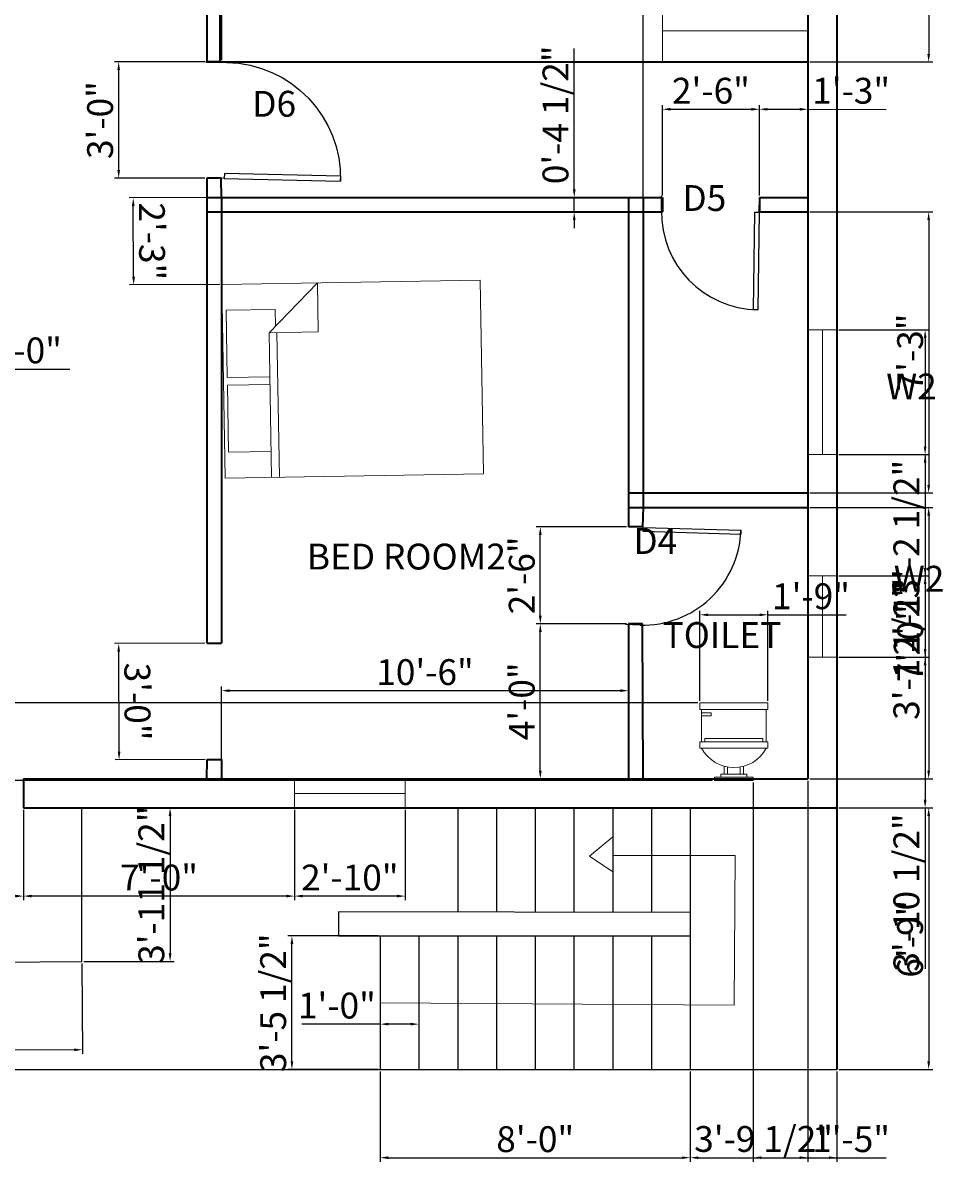
# Model space of a CAD drawing. Units: inches. Extents: x 56 to 631, y 587 to 1198.
# Tile 2 of 3: x 344 to 631, y 587 to 946. Entities that reach past the tile are written whole.
import ezdxf

# ---------------------------------------------------------------- set-up
doc = ezdxf.new("R2010")
doc.units = ezdxf.units.IN
for name, color, linetype, lineweight in [('A-ANNO-DIMS', 2, 'Continuous', 18), ('A-ANNO-SYMB', 2, 'Continuous', 13), ('A-ANNO-TEXT', 7, 'Continuous', 18), ('A-AREA-IDEN', 7, 'Continuous', 25), ('A-DOOR', 3, 'Continuous', 25), ('A-FLOR-CASE', 9, 'Continuous', 18), ('A-FLOR-FIXT', 9, 'Continuous', 18), ('A-FLOR-OTLN', 7, 'Continuous', 25), ('A-FLOR-STRS', 7, 'Continuous', 25), ('A-FURN', 8, 'Continuous', 18), ('A-GLAZ', 4, 'Continuous', 18), ('WALL', 7, 'Continuous', 35)]:
    doc.layers.add(name, color=color, linetype=linetype, lineweight=lineweight)
doc.styles.get("Standard").update_dxf_attribs({"font": 'arial.ttf', "height": 8})
doc.dimstyles.new('ISO-25', dxfattribs={"dimtxt": 2.5, "dimasz": 2.5, "dimexe": 1.25, "dimexo": 0.625, "dimtad": 1, "dimdec": 1, "dimlunit": 3, "dimtxsty": 'Standard', "dimcen": 2.5, "dimadec": 0, "dimazin": 0, "dimtfac": 1, "dimtdec": 1, "dimtmove": 0, "dimatfit": 3, "dimfxl": 1, "dimarcsym": 0})

# ---------------------------------------------------------------- blocks, each defined once
blk = doc.blocks.new('*U2')
for p, q in [((-40, 0), (-40, 6)), ((0, 0), (0, 6))]:
    blk.add_line(p, q)
blk.add_lwpolyline([(0, 0), (0, -40), (-1.75, -40), (-1.75, 0)], close=True)
blk.add_arc((0, 0), 40, 180, 270)
blk = doc.blocks.new('*U3')
for p, q in [((0, 0), (0, -6)), ((40, 0), (40, -6))]:
    blk.add_line(p, q)
blk.add_lwpolyline([(0, 0), (0, 40), (1.75, 40), (1.75, 0)], close=True)
blk.add_arc((0, 0), 40, 0, 90)
blk = doc.blocks.new('Bed - Queen')
for p, q in [((0, -80.00003), (0, 0)), ((0, 0), (59.99999, 0)), ((59.99999, 0), (59.99999, -80.00003)), ((7.99999, -1.2), (28.79998, -1.2)), ((7.99999, -14.4), (7.99999, -1.2)), ((28.79998, -1.2), (28.79998, -14.4)), ((31.19999, -1.2), (51.99999, -1.2)), ((31.19999, -14.4), (31.19999, -1.2)), ((51.99999, -1.2), (51.99999, -16.4)), ((0, -14.4), (44.8, -14.4)), ((44.8, -16.8), (0, -16.8)), ((59.99999, -29.6), (44.8, -14.4)), ((44.8, -14.4), (44.8, -29.6)), ((51.99999, -16.4), (46.79936, -16.4)), ((44.8, -29.6), (59.99999, -29.6)), ((59.99999, -80.00003), (0, -80.00003))]:
    blk.add_line(p, q)
blk = doc.blocks.new('*U10')
for p, q in [((-10, 22), (-10, 12)), ((10, 12), (10, 22)), ((-10, 21), (-7, 21)), ((-7, 20), (-10, 20)), ((-7, 21), (-7, 20)), ((10.5, 12), (-10.5, 12)), ((-10.5, 10), (-10.5, 12)), ((9, 13), (-9, 13)), ((-9, 13), (-9, 12)), ((9, 12), (9, 13)), ((10.5, 12), (10.5, 10)), ((10.5, 10), (-10.5, 10)), ((-3, 4.4065), (-3, 2)), ((-2, 2), (-2, 4.1658)), ((2, 4.1658), (2, 2)), ((3, 2), (3, 4.4065)), ((4, 2), (-4, 2)), ((-4, 2), (-4, 1)), ((4, 1), (4, 2))]:
    blk.add_line(p, q)
for points in [[(10.5, 22), (10.5, 24), (-10.5, 24), (-10.5, 22)], [(6, 0), (6, 1), (-6, 1), (-6, 0)]]:
    blk.add_lwpolyline(points, close=True)
blk.add_arc((0, 15.3333), 11.3333, 208.0725, 331.9275)
blk = doc.blocks.new('*D17')
at = {"layer": 'A-ANNO-DIMS', "color": 0, "lineweight": -2, "transparency": 16777216}
for p, q in [((211.72, 847), (211.72, 837.38)), ((271.72, 847), (271.72, 837.38)), ((214.22, 838.63), (269.22, 838.63)), ((271.72, 838.63), (358.5, 838.63))]:
    blk.add_line(p, q, dxfattribs=at)
at = {"layer": 'A-ANNO-DIMS', "color": 0, "transparency": 16777216}
for points in [[(214.22, 839.05), (214.22, 838.21), (211.72, 838.63)], [(269.22, 839.05), (269.22, 838.21), (271.72, 838.63)]]:
    blk.add_solid(points, dxfattribs=at)
at = {"layer": 'Defpoints', "color": 0, "transparency": 16777216}
for p in [(211.72, 847.63), (271.72, 847.63), (271.72, 838.63)]:
    blk.add_point(p, dxfattribs=at)
at = {"layer": 'A-ANNO-DIMS', "color": 0, "transparency": 16777216, "insert": (316.36, 843.39), "char_height": 8, "attachment_point": 5}
blk.add_mtext('LOVESEAT 5\'-0"', dxfattribs=at)
blk = doc.blocks.new('*D24')
at = {"layer": 'A-ANNO-DIMS', "color": 0, "lineweight": -2, "transparency": 16777216}
for p, q in [((405.55, 934.28), (405.54, 962.2)), ((408.04, 960.95), (584.4, 961.04)), ((586.91, 934.37), (586.9, 962.3))]:
    blk.add_line(p, q, dxfattribs=at)
at = {"layer": 'A-ANNO-DIMS', "color": 0, "transparency": 16777216}
for points in [[(408.04, 961.37), (408.04, 960.54), (405.54, 960.95)], [(584.4, 961.46), (584.4, 960.63), (586.9, 961.05)]]:
    blk.add_solid(points, dxfattribs=at)
at = {"layer": 'Defpoints', "color": 0, "transparency": 16777216}
for p in [(586.9, 961.05), (405.55, 933.65), (586.92, 933.75)]:
    blk.add_point(p, dxfattribs=at)
at = {"layer": 'A-ANNO-DIMS', "color": 0, "transparency": 16777216, "insert": (496.22, 965.76), "char_height": 8, "attachment_point": 5, "rotation": 0.0297}
blk.add_mtext('15\'-1 1/2"', dxfattribs=at)
blk = doc.blocks.new('*D25')
at = {"layer": 'A-ANNO-DIMS', "color": 0, "lineweight": -2, "transparency": 16777216}
for p, q in [((405.42, 712.41), (405.42, 740.34)), ((407.92, 739.09), (528.92, 739.09)), ((531.42, 712.41), (531.42, 740.34))]:
    blk.add_line(p, q, dxfattribs=at)
at = {"layer": 'A-ANNO-DIMS', "color": 0, "transparency": 16777216}
for points in [[(407.92, 739.5), (407.92, 738.67), (405.42, 739.09)], [(528.92, 739.5), (528.92, 738.67), (531.42, 739.09)]]:
    blk.add_solid(points, dxfattribs=at)
at = {"layer": 'Defpoints', "color": 0, "transparency": 16777216}
for p in [(531.42, 739.09), (405.42, 711.79), (531.42, 711.79)]:
    blk.add_point(p, dxfattribs=at)
at = {"layer": 'A-ANNO-DIMS', "color": 0, "transparency": 16777216, "insert": (468.42, 743.79), "char_height": 8, "attachment_point": 5}
blk.add_mtext('10\'-6"', dxfattribs=at)
blk = doc.blocks.new('*D26')
at = {"layer": 'A-ANNO-DIMS', "color": 0, "lineweight": -2, "transparency": 16777216}
for p, q in [((535.92, 796.41), (535.92, 1113.84)), ((538.42, 1112.59), (584.42, 1112.59)), ((586.92, 796.41), (586.92, 1113.84))]:
    blk.add_line(p, q, dxfattribs=at)
at = {"layer": 'A-ANNO-DIMS', "color": 0, "transparency": 16777216}
for points in [[(538.42, 1113), (538.42, 1112.17), (535.92, 1112.59)], [(584.42, 1113), (584.42, 1112.17), (586.92, 1112.59)]]:
    blk.add_solid(points, dxfattribs=at)
at = {"layer": 'Defpoints', "color": 0, "transparency": 16777216}
for p in [(586.92, 1112.59), (535.92, 795.79), (586.92, 795.79)]:
    blk.add_point(p, dxfattribs=at)
at = {"layer": 'A-ANNO-DIMS', "color": 0, "transparency": 16777216, "insert": (561.42, 1117.3), "char_height": 8, "attachment_point": 5}
blk.add_mtext('4\'-3"', dxfattribs=at)
blk = doc.blocks.new('*D29')
at = {"layer": 'A-ANNO-DIMS', "color": 0, "lineweight": -2, "transparency": 16777216}
for p, q in [((596.54, 702.79), (625.57, 702.79)), ((624.32, 700.29), (624.32, 624.29)), ((596.54, 621.79), (625.57, 621.79))]:
    blk.add_line(p, q, dxfattribs=at)
at = {"layer": 'A-ANNO-DIMS', "color": 0, "transparency": 16777216}
for points in [[(623.9, 700.29), (624.74, 700.29), (624.32, 702.79)], [(623.9, 624.29), (624.74, 624.29), (624.32, 621.79)]]:
    blk.add_solid(points, dxfattribs=at)
at = {"layer": 'Defpoints', "color": 0, "transparency": 16777216}
for p in [(595.92, 702.79), (595.92, 621.79), (624.32, 621.79)]:
    blk.add_point(p, dxfattribs=at)
at = {"layer": 'A-ANNO-DIMS', "color": 0, "transparency": 16777216, "insert": (619.61, 662.29), "char_height": 8, "attachment_point": 5, "rotation": 90}
blk.add_mtext('6\'-9"', dxfattribs=at)
blk = doc.blocks.new('*D30')
at = {"layer": 'A-ANNO-DIMS', "color": 0, "lineweight": -2, "transparency": 16777216}
for p, q in [((587.54, 1076.29), (625.57, 1076.29)), ((624.32, 1073.79), (624.32, 936.25)), ((587.54, 933.75), (625.57, 933.75))]:
    blk.add_line(p, q, dxfattribs=at)
at = {"layer": 'A-ANNO-DIMS', "color": 0, "transparency": 16777216}
for points in [[(623.9, 1073.79), (624.74, 1073.79), (624.32, 1076.29)], [(623.9, 936.25), (624.74, 936.25), (624.32, 933.75)]]:
    blk.add_solid(points, dxfattribs=at)
at = {"layer": 'Defpoints', "color": 0, "transparency": 16777216}
for p in [(586.92, 1076.29), (586.92, 933.75), (624.32, 933.75)]:
    blk.add_point(p, dxfattribs=at)
at = {"layer": 'A-ANNO-DIMS', "color": 0, "transparency": 16777216, "insert": (619.56, 1005.02), "char_height": 8, "attachment_point": 5, "rotation": 90}
blk.add_mtext('11\'-10 1/2"', dxfattribs=at)
blk = doc.blocks.new('*D31')
at = {"layer": 'A-ANNO-DIMS', "color": 0, "lineweight": -2, "transparency": 16777216}
for p, q in [((587.54, 887.29), (625.57, 887.29)), ((624.32, 884.79), (624.32, 802.79)), ((587.54, 800.29), (625.57, 800.29))]:
    blk.add_line(p, q, dxfattribs=at)
at = {"layer": 'A-ANNO-DIMS', "color": 0, "transparency": 16777216}
for points in [[(623.9, 884.79), (624.74, 884.79), (624.32, 887.29)], [(623.9, 802.79), (624.74, 802.79), (624.32, 800.29)]]:
    blk.add_solid(points, dxfattribs=at)
at = {"layer": 'Defpoints', "color": 0, "transparency": 16777216}
for p in [(586.92, 887.29), (586.92, 800.29), (624.32, 800.29)]:
    blk.add_point(p, dxfattribs=at)
at = {"layer": 'A-ANNO-DIMS', "color": 0, "transparency": 16777216, "insert": (619.61, 843.79), "char_height": 8, "attachment_point": 5, "rotation": 90}
blk.add_mtext('7\'-3"', dxfattribs=at)
blk = doc.blocks.new('*D32')
at = {"layer": 'A-ANNO-DIMS', "color": 0, "lineweight": -2, "transparency": 16777216}
for p, q in [((587.54, 795.79), (625.57, 795.79)), ((624.32, 793.29), (624.32, 714.29)), ((587.54, 711.79), (625.57, 711.79))]:
    blk.add_line(p, q, dxfattribs=at)
at = {"layer": 'A-ANNO-DIMS', "color": 0, "transparency": 16777216}
for points in [[(623.9, 793.29), (624.74, 793.29), (624.32, 795.79)], [(623.9, 714.29), (624.74, 714.29), (624.32, 711.79)]]:
    blk.add_solid(points, dxfattribs=at)
at = {"layer": 'Defpoints', "color": 0, "transparency": 16777216}
for p in [(586.92, 795.79), (586.92, 711.79), (624.32, 711.79)]:
    blk.add_point(p, dxfattribs=at)
at = {"layer": 'A-ANNO-DIMS', "color": 0, "transparency": 16777216, "insert": (619.61, 753.79), "char_height": 8, "attachment_point": 5, "rotation": 90}
blk.add_mtext('7\'-0"', dxfattribs=at)
blk = doc.blocks.new('*D40')
at = {"layer": 'A-ANNO-DIMS', "color": 0, "lineweight": -2, "transparency": 16777216}
for p, q in [((296.18, 702.16), (296.18, 674.24)), ((344.18, 702.16), (344.18, 674.24)), ((341.68, 675.49), (298.68, 675.49))]:
    blk.add_line(p, q, dxfattribs=at)
at = {"layer": 'A-ANNO-DIMS', "color": 0, "transparency": 16777216}
for points in [[(298.68, 675.9), (298.68, 675.07), (296.18, 675.49)], [(341.68, 675.9), (341.68, 675.07), (344.18, 675.49)]]:
    blk.add_solid(points, dxfattribs=at)
at = {"layer": 'Defpoints', "color": 0, "transparency": 16777216}
for p in [(296.18, 702.79), (344.18, 702.79), (296.18, 675.49)]:
    blk.add_point(p, dxfattribs=at)
at = {"layer": 'A-ANNO-DIMS', "color": 0, "transparency": 16777216, "insert": (320.18, 680.19), "char_height": 8, "attachment_point": 5}
blk.add_mtext('4\'-0"', dxfattribs=at)
blk = doc.blocks.new('*D41')
at = {"layer": 'A-ANNO-DIMS', "color": 0, "lineweight": -2, "transparency": 16777216}
for p, q in [((344.18, 702.16), (344.18, 674.24)), ((428.03, 702.16), (428.03, 674.24)), ((425.53, 675.49), (346.68, 675.49))]:
    blk.add_line(p, q, dxfattribs=at)
at = {"layer": 'A-ANNO-DIMS', "color": 0, "transparency": 16777216}
for points in [[(346.68, 675.9), (346.68, 675.07), (344.18, 675.49)], [(425.53, 675.9), (425.53, 675.07), (428.03, 675.49)]]:
    blk.add_solid(points, dxfattribs=at)
at = {"layer": 'Defpoints', "color": 0, "transparency": 16777216}
for p in [(344.18, 702.79), (428.03, 702.79), (344.18, 675.49)]:
    blk.add_point(p, dxfattribs=at)
at = {"layer": 'A-ANNO-DIMS', "color": 0, "transparency": 16777216, "insert": (386.11, 680.19), "char_height": 8, "attachment_point": 5}
blk.add_mtext('7\'-0"', dxfattribs=at)
blk = doc.blocks.new('*D42')
at = {"layer": 'A-ANNO-DIMS', "color": 0, "lineweight": -2, "transparency": 16777216}
for p, q in [((428.03, 702.16), (428.03, 674.24)), ((462.27, 702.16), (462.27, 674.24)), ((459.77, 675.49), (430.53, 675.49))]:
    blk.add_line(p, q, dxfattribs=at)
at = {"layer": 'A-ANNO-DIMS', "color": 0, "transparency": 16777216}
for points in [[(430.53, 675.9), (430.53, 675.07), (428.03, 675.49)], [(459.77, 675.9), (459.77, 675.07), (462.27, 675.49)]]:
    blk.add_solid(points, dxfattribs=at)
at = {"layer": 'Defpoints', "color": 0, "transparency": 16777216}
for p in [(428.03, 702.79), (462.27, 702.79), (428.03, 675.49)]:
    blk.add_point(p, dxfattribs=at)
at = {"layer": 'A-ANNO-DIMS', "color": 0, "transparency": 16777216, "insert": (445.15, 680.19), "char_height": 8, "attachment_point": 5}
blk.add_mtext('2\'-10"', dxfattribs=at)
blk = doc.blocks.new('*D51')
at = {"layer": 'A-ANNO-DIMS', "color": 0, "lineweight": -2, "transparency": 16777216}
for p, q in [((596.54, 774.6), (624.47, 774.6)), ((623.22, 772.1), (623.22, 751.96)), ((596.54, 749.46), (624.47, 749.46))]:
    blk.add_line(p, q, dxfattribs=at)
at = {"layer": 'A-ANNO-DIMS', "color": 0, "transparency": 16777216}
for points in [[(622.8, 772.1), (623.63, 772.1), (623.22, 774.6)], [(622.8, 751.96), (623.63, 751.96), (623.22, 749.46)]]:
    blk.add_solid(points, dxfattribs=at)
at = {"layer": 'Defpoints', "color": 0, "transparency": 16777216}
for p in [(595.92, 774.6), (595.92, 749.46), (623.22, 749.46)]:
    blk.add_point(p, dxfattribs=at)
at = {"layer": 'A-ANNO-DIMS', "color": 0, "transparency": 16777216, "insert": (618.57, 762.03), "char_height": 8, "attachment_point": 5, "rotation": 90}
blk.add_mtext('2\'-1"', dxfattribs=at)
blk = doc.blocks.new('*D52')
at = {"layer": 'A-ANNO-DIMS', "color": 0, "lineweight": -2, "transparency": 16777216}
for p, q in [((596.54, 749.46), (624.47, 749.46)), ((623.22, 746.96), (623.22, 705.29)), ((596.54, 702.79), (624.47, 702.79)), ((623.22, 702.79), (623.22, 652.92))]:
    blk.add_line(p, q, dxfattribs=at)
at = {"layer": 'A-ANNO-DIMS', "color": 0, "transparency": 16777216}
for points in [[(622.8, 746.96), (623.63, 746.96), (623.22, 749.46)], [(622.8, 705.29), (623.63, 705.29), (623.22, 702.79)]]:
    blk.add_solid(points, dxfattribs=at)
at = {"layer": 'Defpoints', "color": 0, "transparency": 16777216}
for p in [(595.92, 749.46), (595.92, 702.79), (623.22, 702.79)]:
    blk.add_point(p, dxfattribs=at)
at = {"layer": 'A-ANNO-DIMS', "color": 0, "transparency": 16777216, "insert": (618.45, 676.6), "char_height": 8, "attachment_point": 5, "rotation": 90}
blk.add_mtext('3\'-10 1/2"', dxfattribs=at)
blk = doc.blocks.new('*D53')
at = {"layer": 'A-ANNO-DIMS', "color": 0, "lineweight": -2, "transparency": 16777216}
for p, q in [((596.54, 812.18), (624.47, 812.18)), ((623.22, 809.68), (623.22, 777.1)), ((596.54, 774.6), (624.47, 774.6)), ((623.22, 774.6), (623.22, 730.95))]:
    blk.add_line(p, q, dxfattribs=at)
at = {"layer": 'A-ANNO-DIMS', "color": 0, "transparency": 16777216}
for points in [[(622.8, 809.68), (623.63, 809.68), (623.22, 812.18)], [(622.8, 777.1), (623.63, 777.1), (623.22, 774.6)]]:
    blk.add_solid(points, dxfattribs=at)
at = {"layer": 'Defpoints', "color": 0, "transparency": 16777216}
for p in [(595.92, 812.18), (595.92, 774.6), (623.22, 774.6)]:
    blk.add_point(p, dxfattribs=at)
at = {"layer": 'A-ANNO-DIMS', "color": 0, "transparency": 16777216, "insert": (618.45, 751.53), "char_height": 8, "attachment_point": 5, "rotation": 90}
blk.add_mtext('3\'-1 1/2"', dxfattribs=at)
blk = doc.blocks.new('*D54')
at = {"layer": 'A-ANNO-DIMS', "color": 0, "lineweight": -2, "transparency": 16777216}
for p, q in [((596.54, 850.81), (624.47, 850.81)), ((623.22, 848.31), (623.22, 814.68)), ((596.54, 812.18), (624.47, 812.18)), ((623.22, 812.18), (623.22, 768.52))]:
    blk.add_line(p, q, dxfattribs=at)
at = {"layer": 'A-ANNO-DIMS', "color": 0, "transparency": 16777216}
for points in [[(622.8, 848.31), (623.63, 848.31), (623.22, 850.81)], [(622.8, 814.68), (623.63, 814.68), (623.22, 812.18)]]:
    blk.add_solid(points, dxfattribs=at)
at = {"layer": 'Defpoints', "color": 0, "transparency": 16777216}
for p in [(595.92, 850.81), (595.92, 812.18), (623.22, 812.18)]:
    blk.add_point(p, dxfattribs=at)
at = {"layer": 'A-ANNO-DIMS', "color": 0, "transparency": 16777216, "insert": (618.45, 789.1), "char_height": 8, "attachment_point": 5, "rotation": 90}
blk.add_mtext('3\'-2 1/2"', dxfattribs=at)
blk = doc.blocks.new('*D55')
at = {"layer": 'A-ANNO-DIMS', "color": 0, "lineweight": -2, "transparency": 16777216}
for p, q in [((541.92, 892.42), (541.92, 920.34)), ((544.42, 919.09), (569.42, 919.09)), ((571.92, 892.42), (571.92, 920.34))]:
    blk.add_line(p, q, dxfattribs=at)
at = {"layer": 'A-ANNO-DIMS', "color": 0, "transparency": 16777216}
for points in [[(544.42, 919.51), (544.42, 918.68), (541.92, 919.09)], [(569.42, 919.51), (569.42, 918.68), (571.92, 919.09)]]:
    blk.add_solid(points, dxfattribs=at)
at = {"layer": 'Defpoints', "color": 0, "transparency": 16777216}
for p in [(571.92, 919.09), (541.92, 891.79), (571.92, 891.79)]:
    blk.add_point(p, dxfattribs=at)
at = {"layer": 'A-ANNO-DIMS', "color": 0, "transparency": 16777216, "insert": (556.92, 923.8), "char_height": 8, "attachment_point": 5}
blk.add_mtext('2\'-6"', dxfattribs=at)
blk = doc.blocks.new('*D56')
at = {"layer": 'A-ANNO-DIMS', "color": 0, "lineweight": -2, "transparency": 16777216}
for p, q in [((571.92, 892.42), (571.93, 920.34)), ((574.43, 919.09), (584.43, 919.09)), ((586.92, 892.41), (586.93, 920.34)), ((586.93, 919.09), (611.19, 919.07))]:
    blk.add_line(p, q, dxfattribs=at)
at = {"layer": 'A-ANNO-DIMS', "color": 0, "transparency": 16777216}
for points in [[(574.43, 919.51), (574.43, 918.68), (571.93, 919.09)], [(584.43, 919.5), (584.43, 918.67), (586.93, 919.09)]]:
    blk.add_solid(points, dxfattribs=at)
at = {"layer": 'Defpoints', "color": 0, "transparency": 16777216}
for p in [(586.93, 919.09), (571.92, 891.79), (586.92, 891.79)]:
    blk.add_point(p, dxfattribs=at)
at = {"layer": 'A-ANNO-DIMS', "color": 0, "transparency": 16777216, "insert": (600.32, 923.79), "char_height": 8, "attachment_point": 5, "rotation": 359.9661}
blk.add_mtext('1\'-3"', dxfattribs=at)
blk = doc.blocks.new('*D57')
at = {"layer": 'A-ANNO-DIMS', "color": 0, "lineweight": -2, "transparency": 16777216}
for p, q in [((530.79, 789.79), (502.87, 789.79)), ((504.12, 762.29), (504.12, 787.29)), ((530.79, 759.79), (502.87, 759.79))]:
    blk.add_line(p, q, dxfattribs=at)
at = {"layer": 'A-ANNO-DIMS', "color": 0, "transparency": 16777216}
for points in [[(503.7, 787.29), (504.53, 787.29), (504.12, 789.79)], [(503.7, 762.29), (504.53, 762.29), (504.12, 759.79)]]:
    blk.add_solid(points, dxfattribs=at)
at = {"layer": 'Defpoints', "color": 0, "transparency": 16777216}
for p in [(504.12, 789.79), (531.42, 789.79), (531.42, 759.79)]:
    blk.add_point(p, dxfattribs=at)
at = {"layer": 'A-ANNO-DIMS', "color": 0, "transparency": 16777216, "insert": (499.41, 774.79), "char_height": 8, "attachment_point": 5, "rotation": 90}
blk.add_mtext('2\'-6"', dxfattribs=at)
blk = doc.blocks.new('*D58')
at = {"layer": 'A-ANNO-DIMS', "color": 0, "lineweight": -2, "transparency": 16777216}
for p, q in [((530.79, 759.79), (502.87, 759.79)), ((504.12, 714.29), (504.12, 757.29)), ((530.79, 711.79), (502.87, 711.79))]:
    blk.add_line(p, q, dxfattribs=at)
at = {"layer": 'A-ANNO-DIMS', "color": 0, "transparency": 16777216}
for points in [[(503.7, 757.29), (504.53, 757.29), (504.12, 759.79)], [(503.7, 714.29), (504.53, 714.29), (504.12, 711.79)]]:
    blk.add_solid(points, dxfattribs=at)
at = {"layer": 'Defpoints', "color": 0, "transparency": 16777216}
for p in [(504.12, 759.79), (531.42, 759.79), (531.42, 711.79)]:
    blk.add_point(p, dxfattribs=at)
at = {"layer": 'A-ANNO-DIMS', "color": 0, "transparency": 16777216, "insert": (499.41, 735.79), "char_height": 8, "attachment_point": 5, "rotation": 90}
blk.add_mtext('4\'-0"', dxfattribs=at)
blk = doc.blocks.new('*D59')
at = {"layer": 'A-ANNO-DIMS', "color": 0, "lineweight": -2, "transparency": 16777216}
for p, q in [((400.29, 933.75), (372.37, 933.75)), ((373.62, 900.25), (373.62, 931.25)), ((400.29, 897.75), (372.37, 897.75))]:
    blk.add_line(p, q, dxfattribs=at)
at = {"layer": 'A-ANNO-DIMS', "color": 0, "transparency": 16777216}
for points in [[(373.2, 931.25), (374.03, 931.25), (373.62, 933.75)], [(373.2, 900.25), (374.03, 900.25), (373.62, 897.75)]]:
    blk.add_solid(points, dxfattribs=at)
at = {"layer": 'Defpoints', "color": 0, "transparency": 16777216}
for p in [(373.62, 933.75), (400.92, 933.75), (400.92, 897.75)]:
    blk.add_point(p, dxfattribs=at)
at = {"layer": 'A-ANNO-DIMS', "color": 0, "transparency": 16777216, "insert": (368.9, 915.75), "char_height": 8, "attachment_point": 5, "rotation": 90}
blk.add_mtext('3\'-0"', dxfattribs=at)
blk = doc.blocks.new('*D61')
at = {"layer": 'A-ANNO-DIMS', "color": 0, "lineweight": -2, "transparency": 16777216}
for p, q in [((400.29, 753.78), (372.37, 753.68)), ((373.74, 720.18), (373.62, 751.18)), ((400.42, 717.78), (372.5, 717.68))]:
    blk.add_line(p, q, dxfattribs=at)
at = {"layer": 'A-ANNO-DIMS', "color": 0, "transparency": 16777216}
for points in [[(374.04, 751.18), (373.21, 751.18), (373.62, 753.68)], [(374.16, 720.18), (373.32, 720.18), (373.75, 717.68)]]:
    blk.add_solid(points, dxfattribs=at)
at = {"layer": 'Defpoints', "color": 0, "transparency": 16777216}
for p in [(373.62, 753.68), (400.92, 753.78), (401.05, 717.78)]:
    blk.add_point(p, dxfattribs=at)
at = {"layer": 'A-ANNO-DIMS', "color": 0, "transparency": 16777216, "insert": (378.39, 735.7), "char_height": 8, "attachment_point": 5, "rotation": 270.2122}
blk.add_mtext('3\'-0"', dxfattribs=at)
blk = doc.blocks.new('*D62')
at = {"layer": 'A-ANNO-DIMS', "color": 0, "lineweight": -2, "transparency": 16777216}
for p, q in [((454.54, 621.16), (454.54, 593.24)), ((550.54, 621.16), (550.54, 593.24)), ((457.04, 594.49), (548.04, 594.49))]:
    blk.add_line(p, q, dxfattribs=at)
at = {"layer": 'A-ANNO-DIMS', "color": 0, "transparency": 16777216}
for points in [[(457.04, 594.9), (457.04, 594.07), (454.54, 594.49)], [(548.04, 594.9), (548.04, 594.07), (550.54, 594.49)]]:
    blk.add_solid(points, dxfattribs=at)
at = {"layer": 'Defpoints', "color": 0, "transparency": 16777216}
for p in [(454.54, 621.79), (550.54, 621.79), (550.54, 594.49)]:
    blk.add_point(p, dxfattribs=at)
at = {"layer": 'A-ANNO-DIMS', "color": 0, "transparency": 16777216, "insert": (502.54, 599.19), "char_height": 8, "attachment_point": 5}
blk.add_mtext('8\'-0"', dxfattribs=at)
blk = doc.blocks.new('*D63')
at = {"layer": 'A-ANNO-DIMS', "color": 0, "lineweight": -2, "transparency": 16777216}
for p, q in [((550.54, 621.16), (550.54, 593.24)), ((595.92, 621.16), (595.92, 593.24)), ((553.04, 594.49), (593.42, 594.49))]:
    blk.add_line(p, q, dxfattribs=at)
at = {"layer": 'A-ANNO-DIMS', "color": 0, "transparency": 16777216}
for points in [[(553.04, 594.9), (553.04, 594.07), (550.54, 594.49)], [(593.42, 594.9), (593.42, 594.07), (595.92, 594.49)]]:
    blk.add_solid(points, dxfattribs=at)
at = {"layer": 'Defpoints', "color": 0, "transparency": 16777216}
for p in [(550.54, 621.79), (595.92, 621.79), (595.92, 594.49)]:
    blk.add_point(p, dxfattribs=at)
at = {"layer": 'A-ANNO-DIMS', "color": 0, "transparency": 16777216, "insert": (573.23, 599.25), "char_height": 8, "attachment_point": 5}
blk.add_mtext('3\'-9 1/2"', dxfattribs=at)
blk = doc.blocks.new('*D64')
at = {"layer": 'A-ANNO-DIMS', "color": 0, "lineweight": -2, "transparency": 16777216}
for p, q in [((454.54, 662.52), (454.54, 634.59)), ((466.54, 662.52), (466.54, 634.59)), ((454.54, 635.84), (430.27, 635.84)), ((464.04, 635.84), (457.04, 635.84))]:
    blk.add_line(p, q, dxfattribs=at)
at = {"layer": 'A-ANNO-DIMS', "color": 0, "transparency": 16777216}
for points in [[(457.04, 636.26), (457.04, 635.43), (454.54, 635.84)], [(464.04, 636.26), (464.04, 635.43), (466.54, 635.84)]]:
    blk.add_solid(points, dxfattribs=at)
at = {"layer": 'Defpoints', "color": 0, "transparency": 16777216}
for p in [(454.54, 663.14), (466.54, 663.14), (454.54, 635.84)]:
    blk.add_point(p, dxfattribs=at)
at = {"layer": 'A-ANNO-DIMS', "color": 0, "transparency": 16777216, "insert": (441.15, 640.55), "char_height": 8, "attachment_point": 5}
blk.add_mtext('1\'-0"', dxfattribs=at)
blk = doc.blocks.new('*D65')
at = {"layer": 'A-ANNO-DIMS', "color": 0, "lineweight": -2, "transparency": 16777216}
for p, q in [((453.91, 663.14), (425.99, 663.14)), ((427.24, 624.29), (427.24, 660.64)), ((453.91, 621.79), (425.99, 621.79))]:
    blk.add_line(p, q, dxfattribs=at)
at = {"layer": 'A-ANNO-DIMS', "color": 0, "transparency": 16777216}
for points in [[(426.82, 660.64), (427.65, 660.64), (427.24, 663.14)], [(426.82, 624.29), (427.65, 624.29), (427.24, 621.79)]]:
    blk.add_solid(points, dxfattribs=at)
at = {"layer": 'Defpoints', "color": 0, "transparency": 16777216}
for p in [(427.24, 663.14), (454.54, 663.14), (454.54, 621.79)]:
    blk.add_point(p, dxfattribs=at)
at = {"layer": 'A-ANNO-DIMS', "color": 0, "transparency": 16777216, "insert": (422.47, 642.46), "char_height": 8, "attachment_point": 5, "rotation": 90}
blk.add_mtext('3\'-5 1/2"', dxfattribs=at)
blk = doc.blocks.new('*D66')
at = {"layer": 'A-ANNO-DIMS', "color": 0, "lineweight": -2, "transparency": 16777216}
for p, q in [((281.39, 654.16), (281.53, 626.24)), ((362.23, 654.59), (362.38, 626.66)), ((359.87, 627.9), (284.03, 627.5))]:
    blk.add_line(p, q, dxfattribs=at)
at = {"layer": 'A-ANNO-DIMS', "color": 0, "transparency": 16777216}
for points in [[(284.02, 627.92), (284.03, 627.08), (281.53, 627.49)], [(359.87, 628.32), (359.87, 627.48), (362.37, 627.91)]]:
    blk.add_solid(points, dxfattribs=at)
at = {"layer": 'Defpoints', "color": 0, "transparency": 16777216}
for p in [(281.38, 654.79), (362.22, 655.21), (281.53, 627.49)]:
    blk.add_point(p, dxfattribs=at)
at = {"layer": 'A-ANNO-DIMS', "color": 0, "transparency": 16777216, "insert": (321.92, 632.41), "char_height": 8, "attachment_point": 5, "rotation": 0.3029}
blk.add_mtext('6\'-9"', dxfattribs=at)
blk = doc.blocks.new('*D67')
at = {"layer": 'A-ANNO-DIMS', "color": 0, "lineweight": -2, "transparency": 16777216}
for p, q in [((362.85, 702.79), (390.77, 702.79)), ((389.52, 700.29), (389.52, 657.71)), ((362.85, 655.21), (390.77, 655.21))]:
    blk.add_line(p, q, dxfattribs=at)
at = {"layer": 'A-ANNO-DIMS', "color": 0, "transparency": 16777216}
for points in [[(389.11, 700.29), (389.94, 700.29), (389.52, 702.79)], [(389.11, 657.71), (389.94, 657.71), (389.52, 655.21)]]:
    blk.add_solid(points, dxfattribs=at)
at = {"layer": 'Defpoints', "color": 0, "transparency": 16777216}
for p in [(362.22, 702.79), (362.22, 655.21), (389.52, 655.21)]:
    blk.add_point(p, dxfattribs=at)
at = {"layer": 'A-ANNO-DIMS', "color": 0, "transparency": 16777216, "insert": (384.76, 679), "char_height": 8, "attachment_point": 5, "rotation": 90}
blk.add_mtext('3\'-11 1/2"', dxfattribs=at)
blk = doc.blocks.new('*D69')
at = {"layer": 'A-ANNO-DIMS', "color": 0, "lineweight": -2, "transparency": 16777216}
for p, q in [((514.62, 894.29), (514.62, 937.95)), ((541.29, 891.79), (513.37, 891.79)), ((514.62, 887.29), (514.62, 891.79)), ((541.29, 887.29), (513.37, 887.29)), ((514.62, 884.79), (514.62, 882.29))]:
    blk.add_line(p, q, dxfattribs=at)
at = {"layer": 'A-ANNO-DIMS', "color": 0, "transparency": 16777216}
for points in [[(514.2, 894.29), (515.03, 894.29), (514.62, 891.79)], [(514.2, 884.79), (515.03, 884.79), (514.62, 887.29)]]:
    blk.add_solid(points, dxfattribs=at)
at = {"layer": 'Defpoints', "color": 0, "transparency": 16777216}
for p in [(514.62, 891.79), (541.92, 891.79), (541.92, 887.29)]:
    blk.add_point(p, dxfattribs=at)
at = {"layer": 'A-ANNO-DIMS', "color": 0, "transparency": 16777216, "insert": (509.85, 917.37), "char_height": 8, "attachment_point": 5, "rotation": 90}
blk.add_mtext('0\'-4 1/2"', dxfattribs=at)
blk = doc.blocks.new('*D76')
at = {"layer": 'A-ANNO-DIMS', "color": 0, "lineweight": -2, "transparency": 16777216}
for p, q in [((404.79, 891.78), (376.87, 891.64)), ((378.24, 867.21), (378.13, 889.15)), ((404.92, 864.85), (377, 864.71))]:
    blk.add_line(p, q, dxfattribs=at)
at = {"layer": 'A-ANNO-DIMS', "color": 0, "transparency": 16777216}
for points in [[(378.54, 889.15), (377.71, 889.15), (378.12, 891.65)], [(378.65, 867.22), (377.82, 867.21), (378.25, 864.71)]]:
    blk.add_solid(points, dxfattribs=at)
at = {"layer": 'Defpoints', "color": 0, "transparency": 16777216}
for p in [(378.12, 891.65), (405.42, 891.79), (405.55, 864.85)]:
    blk.add_point(p, dxfattribs=at)
at = {"layer": 'A-ANNO-DIMS', "color": 0, "transparency": 16777216, "insert": (382.89, 878.21), "char_height": 8, "attachment_point": 5, "rotation": 270.2822}
blk.add_mtext('2\'-3"', dxfattribs=at)
blk = doc.blocks.new('*D78')
at = {"layer": 'A-ANNO-DIMS', "color": 0, "lineweight": -2, "transparency": 16777216}
for p, q in [((553.52, 735.89), (553.52, 763.82)), ((574.52, 735.89), (574.52, 763.82)), ((556.02, 762.57), (572.02, 762.57)), ((574.52, 762.57), (598.78, 762.57))]:
    blk.add_line(p, q, dxfattribs=at)
at = {"layer": 'A-ANNO-DIMS', "color": 0, "transparency": 16777216}
for points in [[(556.02, 762.98), (556.02, 762.15), (553.52, 762.57)], [(572.02, 762.98), (572.02, 762.15), (574.52, 762.57)]]:
    blk.add_solid(points, dxfattribs=at)
at = {"layer": 'Defpoints', "color": 0, "transparency": 16777216}
for p in [(574.52, 762.57), (553.52, 735.27), (574.52, 735.27)]:
    blk.add_point(p, dxfattribs=at)
at = {"layer": 'A-ANNO-DIMS', "color": 0, "transparency": 16777216, "insert": (587.9, 767.28), "char_height": 8, "attachment_point": 5}
blk.add_mtext('1\'-9"', dxfattribs=at)
blk = doc.blocks.new('*D79')
at = {"layer": 'A-ANNO-DIMS', "color": 0, "lineweight": -2, "transparency": 16777216}
for p, q in [((552.89, 735.27), (64.47, 735.27)), ((65.72, 732.77), (65.72, 713.77)), ((557.39, 711.27), (64.47, 711.27))]:
    blk.add_line(p, q, dxfattribs=at)
at = {"layer": 'A-ANNO-DIMS', "color": 0, "transparency": 16777216}
for points in [[(65.31, 732.77), (66.14, 732.77), (65.72, 735.27)], [(65.31, 713.77), (66.14, 713.77), (65.72, 711.27)]]:
    blk.add_solid(points, dxfattribs=at)
at = {"layer": 'Defpoints', "color": 0, "transparency": 16777216}
for p in [(553.52, 735.27), (65.72, 711.27), (558.02, 711.27)]:
    blk.add_point(p, dxfattribs=at)
at = {"layer": 'A-ANNO-DIMS', "color": 0, "transparency": 16777216, "insert": (61.01, 723.27), "char_height": 8, "attachment_point": 5, "rotation": 90}
blk.add_mtext('2\'-0"', dxfattribs=at)
blk = doc.blocks.new('*D80')
at = {"layer": 'A-ANNO-DIMS', "color": 0, "lineweight": -2, "transparency": 16777216}
for p, q in [((570.02, 710.64), (570.02, 593.24)), ((586.92, 711.16), (586.92, 593.24)), ((572.52, 594.49), (584.42, 594.49)), ((586.92, 594.49), (611.18, 594.49))]:
    blk.add_line(p, q, dxfattribs=at)
at = {"layer": 'A-ANNO-DIMS', "color": 0, "transparency": 16777216}
for points in [[(572.52, 594.9), (572.52, 594.07), (570.02, 594.49)], [(584.42, 594.9), (584.42, 594.07), (586.92, 594.49)]]:
    blk.add_solid(points, dxfattribs=at)
at = {"layer": 'Defpoints', "color": 0, "transparency": 16777216}
for p in [(570.02, 711.27), (586.92, 711.79), (586.92, 594.49)]:
    blk.add_point(p, dxfattribs=at)
at = {"layer": 'A-ANNO-DIMS', "color": 0, "transparency": 16777216, "insert": (600.3, 599.19), "char_height": 8, "attachment_point": 5}
blk.add_mtext('1\'-5"', dxfattribs=at)

msp = doc.modelspace()

# ---------------------------------------------------------------- linework, layer by layer
at = {"layer": 'A-ANNO-SYMB'}
for p, q in [((526.54, 693.79), (519.33, 687.88)), ((519.33, 687.88), (526.54, 683.02)), ((564.4, 688.07), (526.54, 688.07)), ((564.08, 641.71), (564.4, 688.07)), ((454.54, 642.46), (564.08, 641.71))]:
    msp.add_line(p, q, dxfattribs=at)
at = {"layer": 'A-FLOR-CASE'}
for p, q in [((541.96, 933.75), (541.96, 1076.29)), ((541.96, 943.37), (586.92, 943.37))]:
    msp.add_line(p, q, dxfattribs=at)
at = {"layer": 'A-FLOR-OTLN'}
msp.add_line((151.92, 621.79), (595.92, 621.79), dxfattribs=at)
at = {"layer": 'A-FLOR-STRS'}
for p, q in [((362.22, 655.21), (362.22, 702.79)), ((478.54, 702.79), (478.54, 670.57)), ((490.54, 702.79), (490.54, 670.54)), ((502.54, 702.79), (502.54, 670.51)), ((514.54, 702.79), (514.54, 670.48)), ((526.54, 702.79), (526.54, 670.46)), ((538.54, 702.79), (538.54, 670.43)), ((550.54, 702.79), (550.54, 621.79)), ((441.66, 670.65), (441.64, 663.14)), ((550.54, 670.4), (441.66, 670.65)), ((441.64, 663.14), (550.54, 663.14)), ((454.54, 663.14), (454.54, 621.79)), ((466.54, 663.14), (466.54, 621.79)), ((478.54, 663.14), (478.54, 621.79)), ((490.54, 663.14), (490.54, 621.79)), ((502.54, 663.14), (502.54, 621.79)), ((514.54, 663.14), (514.54, 621.79)), ((526.54, 663.14), (526.54, 621.79)), ((538.54, 663.14), (538.54, 621.79)), ((281.38, 654.79), (362.22, 655.21))]:
    msp.add_line(p, q, dxfattribs=at)
at = {"layer": 'A-GLAZ'}
for p, q in [((586.92, 850.81), (595.92, 850.81)), ((591.42, 850.81), (591.42, 812.18)), ((595.92, 850.81), (595.92, 812.18)), ((595.92, 812.18), (586.92, 812.18)), ((586.92, 774.6), (595.92, 774.6)), ((591.42, 774.6), (591.42, 749.46)), ((586.92, 749.46), (595.92, 749.46)), ((428.03, 711.79), (428.03, 702.79)), ((462.27, 702.79), (462.27, 711.79)), ((428.03, 707.29), (462.27, 707.29)), ((428.03, 702.79), (462.27, 702.79))]:
    msp.add_line(p, q, dxfattribs=at)
at = {"layer": 'WALL'}
for p, q in [((595.92, 1085.29), (595.92, 621.79)), ((400.92, 1076.29), (400.92, 933.75)), ((405.06, 933.78), (405.06, 1076.29)), ((586.92, 1076.29), (586.92, 711.79)), ((405.06, 933.78), (400.61, 933.75)), ((400.61, 933.75), (586.92, 933.75)), ((405.36, 897.78), (400.92, 897.75)), ((400.92, 897.75), (400.92, 753.78)), ((405.42, 891.79), (405.36, 897.78)), ((400.92, 891.79), (403.92, 891.79)), ((400.92, 891.79), (541.92, 891.79)), ((405.42, 891.79), (405.42, 753.78)), ((531.42, 891.79), (531.42, 789.79)), ((535.92, 891.79), (535.92, 795.79)), ((535.92, 891.79), (541.92, 891.79)), ((541.92, 891.79), (541.92, 887.29)), ((571.92, 891.79), (571.92, 887.29)), ((571.92, 891.79), (586.92, 891.79)), ((583.92, 891.79), (586.92, 891.79)), ((400.92, 887.29), (541.92, 887.29)), ((571.92, 887.29), (586.92, 887.29)), ((531.42, 800.29), (586.92, 800.29)), ((531.42, 795.79), (586.92, 795.79)), ((535.92, 795.79), (535.79, 789.79)), ((535.79, 789.79), (531.42, 789.79)), ((535.79, 759.79), (531.42, 759.79)), ((531.42, 759.79), (531.42, 711.79)), ((535.92, 711.79), (535.79, 759.79)), ((401.05, 753.78), (405.42, 753.78)), ((400.92, 711.79), (401.05, 717.78)), ((401.05, 717.78), (405.42, 717.78)), ((405.42, 717.78), (405.42, 711.79)), ((344.18, 711.79), (344.18, 702.79)), ((344.18, 711.79), (586.92, 711.79)), ((344.18, 711.79), (586.92, 711.79)), ((344.18, 702.79), (595.92, 702.79))]:
    msp.add_line(p, q, dxfattribs=at)

# ---------------------------------------------------------------- block references
at = {"layer": 'A-DOOR'}
for name, p, xscale, yscale, zscale, rotation in [('*U2', (406.31, 897.63), -0.8999999999999996, 0.8999999999999996, 0.8999999999999996, 88.70842365487967), ('*U3', (571.85, 887.26), 0.7564832307793699, 0.7564832307793699, 0.7564832307793699, 179.1291835171663), ('*U3', (535.95, 789.65), 0.7564832307793699, 0.7564832307793699, 0.7564832307793699, 268.2583670343314)]:
    msp.add_blockref(name, p, dxfattribs=dict(at, xscale=xscale, yscale=yscale, zscale=zscale, rotation=rotation))
at = {"layer": 'A-FLOR-FIXT'}
msp.add_blockref('*U10', (564.02, 711.27), dxfattribs=at)
at = {"layer": 'A-FURN', "rotation": 90.95220825659825}
msp.add_blockref('Bed - Queen', (406.55, 804.86), dxfattribs=at)

# ---------------------------------------------------------------- texts
at = {"layer": 'A-ANNO-TEXT'}
for s, p in [('D6', (414.96, 916.79)), ('D5', (548.11, 887.61)), ('W2', (611.18, 829.26)), ('D4', (532.93, 781.41)), ('W2', (613.52, 769.74))]:
    msp.add_text(s, height=8, dxfattribs=at).set_placement(p)
at = {"layer": 'A-AREA-IDEN'}
for s, p in [('BED ROOM2', (431.87, 776.6)), ('TOILET', (541.97, 752.31))]:
    msp.add_text(s, height=8, dxfattribs=at).set_placement(p)

# ---------------------------------------------------------------- dimensions: what is measured, and where the dimension line sits
at = {"layer": 'A-ANNO-DIMS'}
for base, p1, p2, picture, middle in [((586.92, 1112.59), (535.92, 795.79), (586.92, 795.79), '*D26', (561.42, 1117.3)), ((571.92, 919.09), (541.92, 891.79), (571.92, 891.79), '*D55', (556.92, 923.8)), ((574.52, 762.57), (553.52, 735.27), (574.52, 735.27), '*D78', (587.9, 767.28)), ((531.42, 739.09), (405.42, 711.79), (531.42, 711.79), '*D25', (468.42, 743.79)), ((586.92, 594.49), (570.02, 711.27), (586.92, 711.79), '*D80', (600.3, 599.19)), ((550.54, 594.49), (454.54, 621.79), (550.54, 621.79), '*D62', (502.54, 599.19)), ((595.92, 594.49), (550.54, 621.79), (595.92, 621.79), '*D63', (573.23, 599.25))]:
    dim = msp.add_linear_dim(base=base, p1=p1, p2=p2, dimstyle='ISO-25', override={"dimdec": 1, "dimlfac": 1, "dimrnd": 0, "dimzin": 1, "dimdsep": 46, "dimlunit": 4, "dimfrac": 2}, dxfattribs=at)
    dim.commit()
    dim.dimension.update_dxf_attribs({"geometry": picture, "text_midpoint": middle})
for base, p1, p2, angle, picture, middle in [((624.32, 933.75), (586.92, 1076.29), (586.92, 933.75), 90, '*D30', (619.56, 1005.02)), ((586.9, 961.05), (405.55, 933.65), (586.92, 933.75), 0.0297, '*D24', (496.22, 965.76)), ((514.62, 891.79), (541.92, 887.29), (541.92, 891.79), 90, '*D69', (509.85, 917.37)), ((373.62, 933.75), (400.92, 897.75), (400.92, 933.75), 90, '*D59', (368.9, 915.75)), ((586.93, 919.09), (571.92, 891.79), (586.92, 891.79), 359.9661, '*D56', (600.32, 923.79)), ((378.12, 891.65), (405.55, 864.85), (405.42, 891.79), 90.2822, '*D76', (382.89, 878.21)), ((624.32, 800.29), (586.92, 887.29), (586.92, 800.29), 90, '*D31', (619.61, 843.79)), ((623.22, 812.18), (595.92, 850.81), (595.92, 812.18), 270, '*D54', (618.45, 789.1)), ((623.22, 774.6), (595.92, 812.18), (595.92, 774.6), 270, '*D53', (618.45, 751.53)), ((624.32, 711.79), (586.92, 795.79), (586.92, 711.79), 90, '*D32', (619.61, 753.79)), ((504.12, 789.79), (531.42, 759.79), (531.42, 789.79), 90, '*D57', (499.41, 774.79)), ((623.22, 749.46), (595.92, 774.6), (595.92, 749.46), 270, '*D51', (618.57, 762.03)), ((504.12, 759.79), (531.42, 711.79), (531.42, 759.79), 90, '*D58', (499.41, 735.79)), ((373.62, 753.68), (401.05, 717.78), (400.92, 753.78), 90.2122, '*D61', (378.39, 735.7)), ((623.22, 702.79), (595.92, 749.46), (595.92, 702.79), 270, '*D52', (618.45, 676.6)), ((65.72, 711.27), (553.52, 735.27), (558.02, 711.27), 90, '*D79', (61.01, 723.27)), ((296.18, 675.49), (344.18, 702.79), (296.18, 702.79), 180, '*D40', (320.18, 680.19)), ((344.1844, 675.48502), (428.03444, 702.78502), (344.1844, 702.78502), 180, '*D41', (386.10942, 680.1946)), ((389.52, 655.21), (362.22, 702.79), (362.22, 655.21), 270, '*D67', (384.76, 679)), ((428.03, 675.49), (462.27, 702.79), (428.03, 702.79), 180, '*D42', (445.15, 680.19)), ((624.32, 621.79), (595.92, 702.79), (595.92, 621.79), 90, '*D29', (619.61, 662.29)), ((427.2362, 663.1422), (454.5362, 621.785), (454.5362, 663.1422), 90, '*D65', (422.472, 642.4636)), ((454.54, 635.84), (466.54, 663.14), (454.54, 663.14), 180, '*D64', (441.15, 640.55)), ((281.53, 627.49), (362.22, 655.21), (281.38, 654.79), 180.3029, '*D66', (321.92, 632.41))]:
    dim = msp.add_linear_dim(base=base, p1=p1, p2=p2, angle=angle, dimstyle='ISO-25', override={"dimdec": 1, "dimlfac": 1, "dimrnd": 0, "dimzin": 1, "dimdsep": 46, "dimlunit": 4, "dimfrac": 2}, dxfattribs=at)
    dim.commit()
    dim.dimension.update_dxf_attribs({"geometry": picture, "text_midpoint": middle})
dim = msp.add_linear_dim(base=(271.72, 838.63), p1=(211.72, 847.63), p2=(271.72, 847.63), text='LOVESEAT <>', dimstyle='ISO-25', override={"dimdec": 1, "dimlfac": 1, "dimrnd": 0, "dimzin": 1, "dimdsep": 46, "dimlunit": 4, "dimfrac": 2}, dxfattribs=at)
dim.commit()
dim.dimension.update_dxf_attribs({"geometry": '*D17', "text_midpoint": (316.36, 843.39)})

doc.saveas('drawing.dxf')
